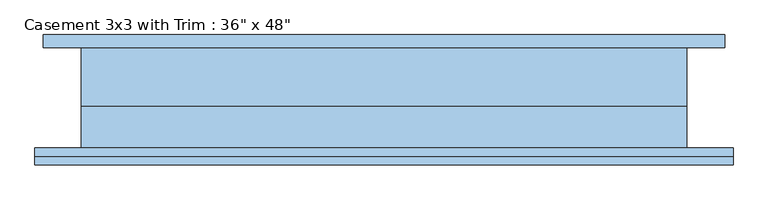
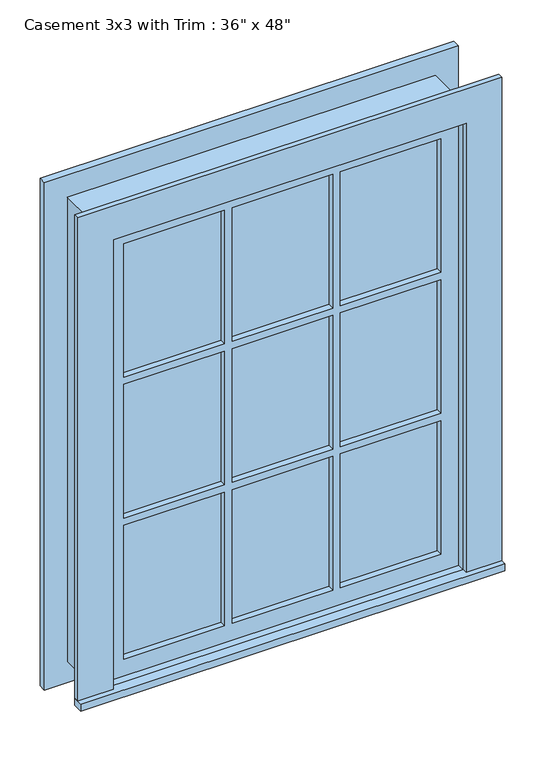
"""IFC4 building model written with IfcOpenShell, lengths in millimetres: window geometry."""

from ifc_helpers import new_model, si_unit, frame, origin, place, context, project, spatial, polyline, outline, extrude, source, transform, mapped, element, save


def window_7947f0f9(model_context):
    return source(origin(), model_context, "Body", "SweptSolid", [
        extrude(outline(polyline([(-527.05, -101.6), (-527.05, -76.2), (527.05, -76.2), (527.05, -101.6), (-527.05, -101.6)])), frame((0.0, 0.0, 914.4), z_axis=(0.0, 0.0, 1.0), x_axis=(1.0, 0.0, 0.0)), (0.0, 0.0, 1.0), 19.05),
        extrude(outline(polyline([(2114.55, -438.15), (2114.55, 438.15), (933.45, 438.15), (933.45, 527.05), (2203.45, 527.05), (2203.45, -527.05), (933.45, -527.05), (933.45, -438.15), (2114.55, -438.15)])), frame((0.0, -88.9, 0.0), z_axis=(0.0, 1.0, 0.0), x_axis=(0.0, 0.0, 1.0)), (0.0, 0.0, 1.0), 12.7),
        extrude(outline(polyline([(143.9333333, -41.275), (143.9333333, -28.575), (393.7, -28.575), (393.7, -41.275), (143.9333333, -41.275)])), frame((0.0, 0.0, 1718.7333333), z_axis=(0.0, 0.0, 1.0), x_axis=(1.0, 0.0, 0.0)), (0.0, 0.0, 1.0), 351.3666667),
        extrude(outline(polyline([(-124.8833333, -41.275), (-124.8833333, -28.575), (124.8833333, -28.575), (124.8833333, -41.275), (-124.8833333, -41.275)])), frame((0.0, 0.0, 1718.7333333), z_axis=(0.0, 0.0, 1.0), x_axis=(1.0, 0.0, 0.0)), (0.0, 0.0, 1.0), 351.3666667),
        extrude(outline(polyline([(-393.7, -41.275), (-393.7, -28.575), (-143.9333333, -28.575), (-143.9333333, -41.275), (-393.7, -41.275)])), frame((0.0, 0.0, 1718.7333333), z_axis=(0.0, 0.0, 1.0), x_axis=(1.0, 0.0, 0.0)), (0.0, 0.0, 1.0), 351.3666667),
        extrude(outline(polyline([(-393.7, -41.275), (-393.7, -28.575), (-143.9333333, -28.575), (-143.9333333, -41.275), (-393.7, -41.275)])), frame((0.0, 0.0, 1348.3166667), z_axis=(0.0, 0.0, 1.0), x_axis=(1.0, 0.0, 0.0)), (0.0, 0.0, 1.0), 351.3666667),
        extrude(outline(polyline([(-124.8833333, -41.275), (-124.8833333, -28.575), (124.8833333, -28.575), (124.8833333, -41.275), (-124.8833333, -41.275)])), frame((0.0, 0.0, 1348.3166667), z_axis=(0.0, 0.0, 1.0), x_axis=(1.0, 0.0, 0.0)), (0.0, 0.0, 1.0), 351.3666667),
        extrude(outline(polyline([(143.9333333, -41.275), (143.9333333, -28.575), (393.7, -28.575), (393.7, -41.275), (143.9333333, -41.275)])), frame((0.0, 0.0, 1348.3166667), z_axis=(0.0, 0.0, 1.0), x_axis=(1.0, 0.0, 0.0)), (0.0, 0.0, 1.0), 351.3666667),
        extrude(outline(polyline([(143.9333333, -41.275), (143.9333333, -28.575), (393.7, -28.575), (393.7, -41.275), (143.9333333, -41.275)])), frame((0.0, 0.0, 977.9), z_axis=(0.0, 0.0, 1.0), x_axis=(1.0, 0.0, 0.0)), (0.0, 0.0, 1.0), 351.3666667),
        extrude(outline(polyline([(-124.8833333, -41.275), (-124.8833333, -28.575), (124.8833333, -28.575), (124.8833333, -41.275), (-124.8833333, -41.275)])), frame((0.0, 0.0, 977.9), z_axis=(0.0, 0.0, 1.0), x_axis=(1.0, 0.0, 0.0)), (0.0, 0.0, 1.0), 351.3666667),
        extrude(outline(polyline([(-393.7, -41.275), (-393.7, -28.575), (-143.9333333, -28.575), (-143.9333333, -41.275), (-393.7, -41.275)])), frame((0.0, 0.0, 977.9), z_axis=(0.0, 0.0, 1.0), x_axis=(1.0, 0.0, 0.0)), (0.0, 0.0, 1.0), 351.3666667),
        extrude(outline(polyline([(2190.75, 514.35), (2190.75, -514.35), (857.25, -514.35), (857.25, 514.35), (2190.75, 514.35)]), holes=[polyline([(2101.85, 425.45), (946.15, 425.45), (946.15, -425.45), (2101.85, -425.45), (2101.85, 425.45)])]), frame((0.0, 76.2, 0.0), z_axis=(0.0, 1.0, 0.0), x_axis=(0.0, 0.0, 1.0)), (0.0, 0.0, 1.0), 19.05),
        extrude(outline(polyline([(2114.55, -438.15), (933.45, -438.15), (933.45, 438.15), (2114.55, 438.15), (2114.55, -438.15)]), holes=[polyline([(2070.1, -143.9333333), (1718.7333333, -143.9333333), (1718.7333333, -393.7), (2070.1, -393.7), (2070.1, -143.9333333)]), polyline([(1699.6833333, -143.9333333), (1348.3166667, -143.9333333), (1348.3166667, -393.7), (1699.6833333, -393.7), (1699.6833333, -143.9333333)]), polyline([(1329.2666667, -143.9333333), (977.9, -143.9333333), (977.9, -393.7), (1329.2666667, -393.7), (1329.2666667, -143.9333333)]), polyline([(2070.1, 124.8833333), (1718.7333333, 124.8833333), (1718.7333333, -124.8833333), (2070.1, -124.8833333), (2070.1, 124.8833333)]), polyline([(1699.6833333, 124.8833333), (1348.3166667, 124.8833333), (1348.3166667, -124.8833333), (1699.6833333, -124.8833333), (1699.6833333, 124.8833333)]), polyline([(1329.2666667, 124.8833333), (977.9, 124.8833333), (977.9, -124.8833333), (1329.2666667, -124.8833333), (1329.2666667, 124.8833333)]), polyline([(2070.1, 393.7), (1718.7333333, 393.7), (1718.7333333, 143.9333333), (2070.1, 143.9333333), (2070.1, 393.7)]), polyline([(1699.6833333, 393.7), (1348.3166667, 393.7), (1348.3166667, 143.9333333), (1699.6833333, 143.9333333), (1699.6833333, 393.7)]), polyline([(1329.2666667, 393.7), (977.9, 393.7), (977.9, 143.9333333), (1329.2666667, 143.9333333), (1329.2666667, 393.7)])]), frame((0.0, -57.15, 0.0), z_axis=(0.0, 1.0, 0.0), x_axis=(0.0, 0.0, 1.0)), (0.0, 0.0, 1.0), 44.45),
        extrude(outline(polyline([(2133.6, -457.2), (914.4, -457.2), (914.4, 457.2), (2133.6, 457.2), (2133.6, -457.2)]), holes=[polyline([(2101.85, -425.45), (2101.85, 425.45), (946.15, 425.45), (946.15, -425.45), (2101.85, -425.45)])]), frame((0.0, -12.7, 0.0), z_axis=(0.0, 1.0, 0.0), x_axis=(0.0, 0.0, 1.0)), (0.0, 0.0, 1.0), 88.9),
        extrude(outline(polyline([(2133.6, 457.2), (2133.6, -457.2), (914.4, -457.2), (914.4, 457.2), (2133.6, 457.2)]), holes=[polyline([(2114.55, 438.15), (933.45, 438.15), (933.45, -438.15), (2114.55, -438.15), (2114.55, 438.15)])]), frame((0.0, -76.2, 0.0), z_axis=(0.0, 1.0, 0.0), x_axis=(0.0, 0.0, 1.0)), (0.0, 0.0, 1.0), 63.5),
    ])


if __name__ == "__main__":
    model = new_model("IFC4")
    model_context = context("Model", 3, world=origin())
    ifc_project = project(units=[si_unit("LENGTHUNIT", "METRE", prefix="MILLI")], contexts=[model_context])
    site = spatial("IfcSite", under=ifc_project)
    building = spatial("IfcBuilding", under=site)
    placement = place(None, origin())
    window_shape = window_7947f0f9(model_context)
    element("IfcWindow", 1, ObjectType="Casement 3x3 with Trim : 36\" x 48\"", at=placement, inside=building, context=model_context, shape_type="MappedRepresentation", body=[
        mapped(window_shape, transform((0.0, 0.0, 0.0), x_axis=(1.0, 0.0, 0.0), y_axis=(0.0, 1.0, 0.0), z_axis=(0.0, 0.0, 1.0))),
    ])
    save(model, "model.ifc")

# Revit data of these elements
# Type "Casement 3x3 with Trim : 36\" x 48\""
#   Type Mark = "10"
#   Construction Type Id = "GSP4R"
#   Assembly Code = "B2020100"
#   Analytic Construction = "1/8 in Pilkington single glazing"
#   Visual Light Transmittance = 0.9
#   Solar Heat Gain Coefficient = 0.78
#   Heat Transfer Coefficient (U) = 0.6496 BTU/(h·ft²·°F)
#   Height = 4' - 0"
#   Default Sill Height = 3' - 0"
#   Trim Projection - Ext. = 0' - 0 1/2"
#   Trim Projection - Int. = 0' - 0 3/4"
#   Trim Width - Exterior = 0' - 3 1/2"
#   Trim Width - Interior = 0' - 3 1/2"
#   Width = 3' - 0"
#   Window Inset = 0' - 0 3/4"
#   Define Thermal Properties by = 1
#   Glass Pane Material = Glass
#   Sash Material = Sash
#   Trim Exterior Material = Trim
#   Trim Interior Material = Trim
#   Wall Closure = (empty or 0)
# Element 1 (IfcWindow, "Casement 3x3 with Trim : 36\" x 48\"")
#   Materials on its faces: "Sash", "Glass", "Trim"
# Materials
#   "Glass": class "Glass", colour RGB 0 128 192, transparency 0.75, Description = "Soda Lime Glass", Cost = 0
#   "Sash": class "Wood", colour RGB 224 178 126, transparency 0
#   "Trim": class "Wood", colour RGB 224 178 126, transparency 0
